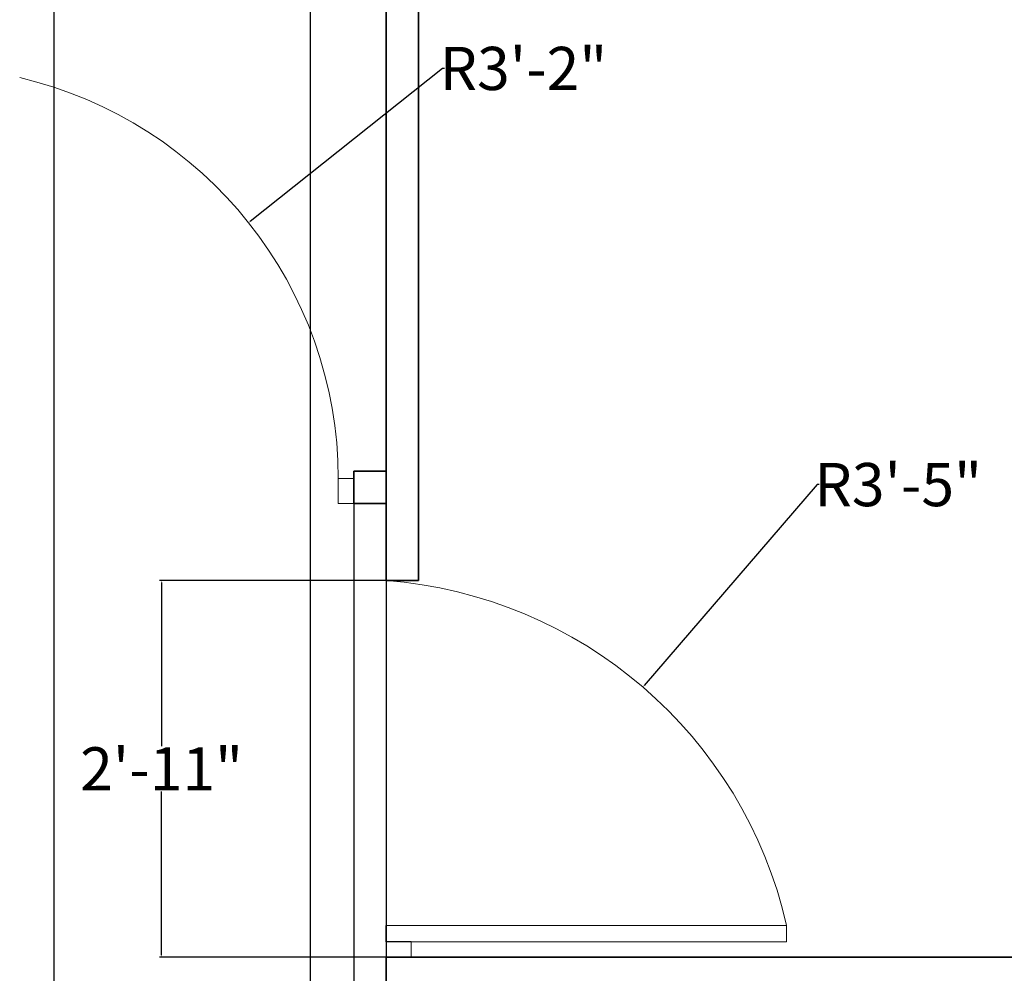
# Model space of a CAD drawing. Units: inches. Extents: x 311 to 754, y 60 to 497.
# Tile 9 of 11: x 530 to 621, y 296 to 384. Entities that reach past the tile are written whole.
import ezdxf

# ---------------------------------------------------------------- set-up
doc = ezdxf.new("R2010")
doc.units = ezdxf.units.IN
doc.header["$MEASUREMENT"] = 0
for name, color, linetype, lineweight in [('A-ANNO-DIMS', 2, 'Continuous', 18), ('A-WALL', 7, 'Continuous', 35), ('beds', 70, 'Continuous', 13), ('doors', 210, 'Continuous', 18)]:
    doc.layers.add(name, color=color, linetype=linetype, lineweight=lineweight)
doc.styles.get("Standard").update_dxf_attribs({"font": 'arial.ttf'})
doc.dimstyles.get("Standard").update_dxf_attribs({"dimtxt": 4, "dimasz": 0.18, "dimexe": 0.18, "dimexo": 0.0625, "dimgap": 0.09, "dimtad": 0, "dimtih": 1, "dimtoh": 1, "dimdec": 0, "dimrnd": 6, "dimzin": 0, "dimdsep": 46, "dimlunit": 3, "dimtxsty": 'Standard', "dimcen": 0.09, "dimadec": 0, "dimazin": 0, "dimtfac": 1, "dimtdec": 0, "dimtofl": 0, "dimtmove": 0, "dimatfit": 3, "dimfxl": 1, "dimtolj": 1, "dimtzin": 0, "dimarcsym": 0})

# ---------------------------------------------------------------- blocks, each defined once
blk = doc.blocks.new('A$C57792D97')
for p, q in [((0.6, 2.6235), (0, 2.6235)), ((0, 2.6235), (0, 2.1735)), ((2.1, 2.6235), (0.6, 2.6235)), ((0.6, 2.6235), (0.6, 0.6235)), ((0.6, 0.6235), (0.6, 2.6235)), ((0.6, 2.1735), (0.6, 2.6235)), ((2.1, 0.6235), (2.1, 2.6235)), ((2.7, 2.6235), (2.1, 2.6235)), ((2.1, 2.6235), (2.1, 2.1735)), ((2.7, 2.1735), (2.7, 2.6235)), ((0.6, 2.5735), (0, 2.5735)), ((2.1, 2.5735), (0.6, 2.5735)), ((2.7, 2.5735), (2.1, 2.5735)), ((2.4103, 2.2312), (2.4103, 2.5317)), ((2.2593, 2.3802), (2.5698, 2.3802)), ((1.5491, 2.1955), (1.5516, 2.1955)), ((0, 2.1735), (0.6, 2.1735)), ((2.1, 2.1735), (2.7, 2.1735)), ((0.6, 2.1518), (0.8661, 2.1518)), ((0.6, 1.9518), (1.4767, 1.9518)), ((0.63, 0.6535), (0.63, 1.9518)), ((0.9906, 1.8942), (0.9508, 1.934)), ((1.4149, 1.8942), (1.3751, 1.934)), ((0.9906, 1.8942), (0.9344, 1.8942)), ((0.9906, 1.8942), (0.9508, 1.8544)), ((1.4149, 1.8942), (1.3586, 1.8942)), ((1.4149, 1.8942), (1.3751, 1.8544)), ((2.142, 1.8959), (2.1018, 1.8254)), ((2.1679, 1.8652), (2.1088, 1.8077)), ((2.1584, 1.8544), (2.1201, 1.8188)), ((2.1812, 1.8524), (2.1207, 1.8046)), ((2.1749, 1.8475), (2.1394, 1.7993)), ((2.2173, 1.8274), (2.1931, 1.7688)), ((2.2496, 1.8292), (2.2008, 1.7642)), ((2.1799, 1.8155), (2.1465, 1.7971)), ((2.2066, 1.8191), (2.1664, 1.7827)), ((2.249, 1.8154), (2.1711, 1.7709)), ((2.2713, 1.7954), (2.2055, 1.7458)), ((2.07, 1.7793), (2.07, 0.6535)), ((2.283, 1.7811), (2.2169, 1.7413)), ((2.2607, 1.7859), (2.2181, 1.7554)), ((2.2761, 1.777), (2.2348, 1.7337)), ((2.277, 1.7446), (2.2416, 1.7306)), ((2.304, 1.7449), (2.2596, 1.7138)), ((2.3456, 1.7359), (2.2627, 1.7015)), ((2.3157, 1.7518), (2.2843, 1.6966)), ((2.3479, 1.7495), (2.2914, 1.6911)), ((0.7785, 1.6821), (0.7387, 1.7219)), ((1.2027, 1.6821), (1.163, 1.7219)), ((1.627, 1.6821), (1.5872, 1.7219)), ((2.0513, 1.6821), (2.0115, 1.7219)), ((2.3653, 1.7133), (2.2937, 1.6723)), ((2.3535, 1.7051), (2.3075, 1.6802)), ((0.7785, 1.6821), (0.7222, 1.6821)), ((0.7785, 1.6821), (0.7387, 1.6423)), ((1.2027, 1.6821), (1.1465, 1.6821)), ((1.2027, 1.6821), (1.163, 1.6423)), ((1.627, 1.6821), (1.5708, 1.6821)), ((1.627, 1.6821), (1.5872, 1.6423)), ((2.0513, 1.6821), (1.995, 1.6821)), ((2.0513, 1.6821), (2.0115, 1.6423)), ((2.3751, 1.6976), (2.3045, 1.6664)), ((2.3677, 1.6944), (2.3213, 1.6565)), ((2.3645, 1.6621), (2.3277, 1.6526)), ((2.3913, 1.659), (2.3434, 1.6337)), ((2.4314, 1.6449), (2.3449, 1.6211)), ((2.4038, 1.6644), (2.3657, 1.6136)), ((2.4355, 1.6581), (2.372, 1.6073)), ((2.4482, 1.62), (2.372, 1.5882)), ((2.4354, 1.6134), (2.3867, 1.5944)), ((2.2754, 1.598), (2.2534, 1.5939)), ((2.2736, 1.5771), (2.2535, 1.594)), ((2.2736, 1.5771), (2.2754, 1.598)), ((2.4559, 1.6032), (2.382, 1.581)), ((2.4482, 1.6009), (2.3974, 1.5692)), ((2.3123, 1.541), (2.2911, 1.5481)), ((2.3006, 1.5236), (2.2912, 1.5481)), ((2.441, 1.5693), (2.4032, 1.5645)), ((2.4672, 1.5629), (2.4164, 1.5438)), ((2.4802, 1.5667), (2.4361, 1.5211)), ((2.5109, 1.5564), (2.4416, 1.514)), ((2.3006, 1.5236), (2.3123, 1.541)), ((2.5052, 1.5438), (2.4164, 1.5311)), ((2.5187, 1.517), (2.4392, 1.4951)), ((0.9906, 1.47), (0.9508, 1.5097)), ((1.4149, 1.47), (1.3751, 1.5097)), ((1.8391, 1.47), (1.7994, 1.5097)), ((2.5243, 1.4994), (2.4482, 1.4867)), ((2.5052, 1.5121), (2.4545, 1.4994)), ((2.5163, 1.4981), (2.462, 1.473)), ((0.9906, 1.47), (0.9344, 1.47)), ((0.9906, 1.47), (0.9508, 1.4302)), ((1.4149, 1.47), (1.3586, 1.47)), ((1.4149, 1.47), (1.3751, 1.4302)), ((1.8391, 1.47), (1.7829, 1.47)), ((1.8391, 1.47), (1.7994, 1.4302)), ((2.5052, 1.4677), (2.4672, 1.4677)), ((2.5304, 1.458), (2.4777, 1.4454)), ((2.5438, 1.4601), (2.4943, 1.4204)), ((2.5658, 1.4343), (2.4761, 1.4328)), ((2.573, 1.4461), (2.4989, 1.4127)), ((2.5758, 1.406), (2.4942, 1.3942)), ((2.5618, 1.4028), (2.5099, 1.3966)), ((2.5791, 1.3878), (2.502, 1.3848)), ((2.571, 1.3876), (2.514, 1.3695)), ((2.1596, 1.3147), (2.1502, 1.3392)), ((2.1714, 1.3321), (2.1502, 1.3392)), ((2.2534, 1.3469), (2.2315, 1.3429)), ((2.2516, 1.326), (2.2315, 1.3429)), ((2.2516, 1.326), (2.2535, 1.347)), ((2.5562, 1.3587), (2.5185, 1.3635)), ((2.58, 1.346), (2.5261, 1.3402)), ((2.5936, 1.3464), (2.5395, 1.3132)), ((2.1596, 1.3147), (2.1714, 1.3321)), ((2.3632, 1.3229), (2.33, 1.319)), ((2.3584, 1.2918), (2.33, 1.319)), ((2.3584, 1.2918), (2.3632, 1.3229)), ((2.6121, 1.3181), (2.523, 1.3279)), ((2.6207, 1.3289), (2.5431, 1.305)), ((0.7785, 1.2578), (0.7387, 1.2976)), ((1.2027, 1.2578), (1.163, 1.2976)), ((1.627, 1.2578), (1.5872, 1.2976)), ((2.0513, 1.2578), (2.0115, 1.2976)), ((2.6185, 1.2888), (2.5361, 1.2873)), ((2.6195, 1.2703), (2.5426, 1.277)), ((2.6042, 1.2873), (2.5519, 1.2877)), ((0.7785, 1.2578), (0.7222, 1.2578)), ((0.7785, 1.2578), (0.7387, 1.218)), ((1.2027, 1.2578), (1.1465, 1.2578)), ((1.2027, 1.2578), (1.163, 1.218)), ((1.627, 1.2578), (1.5708, 1.2578)), ((1.627, 1.2578), (1.5872, 1.218)), ((2.0513, 1.2578), (1.995, 1.2578)), ((2.0513, 1.2578), (2.0115, 1.218)), ((2.4134, 1.2295), (2.404, 1.254)), ((2.4252, 1.2469), (2.404, 1.254)), ((2.4134, 1.2295), (2.4252, 1.2469)), ((2.6115, 1.2711), (2.5526, 1.2603)), ((2.5932, 1.2443), (2.5563, 1.2538)), ((2.6435, 1.197), (2.5563, 1.2178)), ((2.6152, 1.2287), (2.561, 1.2296)), ((2.6287, 1.2274), (2.5709, 1.2013)), ((2.6534, 1.2066), (2.5734, 1.1926)), ((2.6462, 1.1671), (2.5642, 1.176)), ((2.6449, 1.1486), (2.5694, 1.1649)), ((2.6319, 1.1675), (2.58, 1.1743)), ((2.4947, 1.1445), (2.4728, 1.1404)), ((2.4929, 1.1236), (2.4728, 1.1404)), ((2.4929, 1.1236), (2.4948, 1.1445)), ((2.637, 1.1504), (2.5773, 1.147)), ((2.6155, 1.1261), (2.5801, 1.1402)), ((2.2315, 1.0959), (2.2095, 1.0919)), ((2.2297, 1.075), (2.2315, 1.0959)), ((2.6595, 1.0729), (2.5756, 1.1045)), ((2.6353, 1.1079), (2.5817, 1.1156)), ((2.6486, 1.1049), (2.588, 1.0862)), ((0.9906, 1.0457), (0.9508, 1.0855)), ((1.4149, 1.0457), (1.3751, 1.0855)), ((1.8391, 1.0457), (1.7994, 1.0855)), ((2.2297, 1.075), (2.2096, 1.0919)), ((2.6584, 1.0429), (2.5782, 1.062)), ((2.6705, 1.0812), (2.5894, 1.0774)), ((0.9906, 1.0457), (0.9344, 1.0457)), ((0.9906, 1.0457), (0.9508, 1.0059)), ((1.4149, 1.0457), (1.3586, 1.0457)), ((1.4149, 1.0457), (1.3751, 1.0059)), ((1.8391, 1.0457), (1.7829, 1.0457)), ((1.8391, 1.0457), (1.7994, 1.0059)), ((2.2725, 1.0206), (2.2631, 1.0451)), ((2.2842, 1.038), (2.2631, 1.0451)), ((2.2725, 1.0206), (2.2843, 1.038)), ((2.6548, 1.0248), (2.582, 1.0503)), ((2.6472, 1.0275), (2.5875, 1.0316)), ((2.6442, 1.045), (2.5937, 1.0584)), ((2.6228, 1.0061), (2.5895, 1.0244)), ((2.6598, 0.9477), (2.5805, 0.9897)), ((2.6402, 0.9855), (2.588, 0.9999)), ((2.653, 0.9809), (2.5905, 0.97)), ((2.3053, 0.9493), (2.272, 0.9455)), ((2.3005, 0.9182), (2.2721, 0.9455)), ((2.3005, 0.9182), (2.3053, 0.9494)), ((2.5263, 0.9355), (2.5169, 0.96)), ((2.538, 0.9528), (2.5169, 0.9599)), ((2.5263, 0.9355), (2.5381, 0.9529)), ((2.655, 0.9181), (2.5778, 0.9471)), ((2.6718, 0.9546), (2.5908, 0.961)), ((2.6412, 0.9221), (2.5927, 0.9416)), ((2.6491, 0.9006), (2.5801, 0.9351)), ((2.6419, 0.9043), (2.5832, 0.9159)), ((2.4728, 0.8934), (2.4508, 0.8894)), ((2.471, 0.8725), (2.4509, 0.8894)), ((2.471, 0.8725), (2.4728, 0.8934)), ((2.6297, 0.8635), (2.5797, 0.8843)), ((2.6151, 0.8861), (2.5843, 0.9085)), ((0.7785, 0.8336), (0.7387, 0.8733)), ((1.2027, 0.8336), (1.163, 0.8733)), ((1.627, 0.8336), (1.5872, 0.8733)), ((2.0513, 0.8336), (2.0115, 0.8733)), ((2.6444, 0.8236), (2.571, 0.8751)), ((2.6418, 0.8573), (2.5785, 0.8543)), ((0.7785, 0.8336), (0.7222, 0.8336)), ((0.7785, 0.8336), (0.7387, 0.7938)), ((1.2027, 0.8336), (1.1465, 0.8336)), ((1.2027, 0.8336), (1.163, 0.7938)), ((1.627, 0.8336), (1.5708, 0.8336)), ((1.627, 0.8336), (1.5872, 0.7938)), ((2.0513, 0.8336), (1.995, 0.8336)), ((2.0513, 0.8336), (2.0115, 0.7938)), ((2.1316, 0.8117), (2.1222, 0.8362)), ((2.1433, 0.8291), (2.1222, 0.8362)), ((2.1316, 0.8117), (2.1434, 0.8291)), ((2.2095, 0.8449), (2.1876, 0.8408)), ((2.2077, 0.824), (2.1876, 0.8408)), ((2.2077, 0.824), (2.2095, 0.8449)), ((2.6359, 0.7948), (2.5629, 0.8332)), ((2.6279, 0.7781), (2.5637, 0.821)), ((2.6227, 0.8004), (2.577, 0.8259)), ((2.6572, 0.8289), (2.5776, 0.8454)), ((1.9462, 0.7963), (1.9243, 0.7923)), ((2.6212, 0.7827), (2.5644, 0.8015)), ((2.5923, 0.768), (2.5646, 0.7941)), ((2.6136, 0.7023), (2.5472, 0.7626)), ((2.604, 0.7437), (2.557, 0.7707)), ((1.683, 0.7477), (1.661, 0.7437)), ((2.3854, 0.7265), (2.376, 0.751)), ((2.3971, 0.7439), (2.376, 0.751)), ((2.3854, 0.7265), (2.3972, 0.7439)), ((2.6269, 0.706), (2.5501, 0.7323)), ((2.6153, 0.7361), (2.552, 0.7411)), ((1.4197, 0.6992), (1.3978, 0.6951)), ((2.5915, 0.6593), (2.5332, 0.7099)), ((2.6016, 0.6748), (2.534, 0.7221)), ((2.5892, 0.6821), (2.547, 0.7131)), ((2.5549, 0.6537), (2.5307, 0.6831)), ((2.5855, 0.6646), (2.5315, 0.6905)), ((0.9906, 0.6214), (0.9508, 0.6612)), ((1.1564, 0.6506), (1.1345, 0.6466)), ((1.4149, 0.6214), (1.3751, 0.6612)), ((1.8391, 0.6214), (1.7994, 0.6612)), ((2.4508, 0.6424), (2.4289, 0.6383)), ((2.449, 0.6215), (2.4289, 0.6384)), ((2.449, 0.6215), (2.4508, 0.6424)), ((2.5678, 0.5858), (2.5095, 0.654)), ((2.5635, 0.6282), (2.5203, 0.6608)), ((0.9906, 0.6214), (0.9344, 0.6214)), ((0.9906, 0.6214), (0.9727, 0.6035)), ((1.4149, 0.6214), (1.3586, 0.6214)), ((1.4149, 0.6214), (1.397, 0.6035)), ((1.8391, 0.6214), (1.7829, 0.6214)), ((1.8391, 0.6214), (1.8212, 0.6035)), ((2.5524, 0.5601), (2.4913, 0.6155)), ((2.5815, 0.5878), (2.5085, 0.6236)), ((2.5737, 0.6192), (2.5116, 0.632)), ((2.02, 0.6035), (0.6716, 0.6035)), ((0.8932, 0.6021), (0.8712, 0.598)), ((2.1875, 0.5938), (2.1656, 0.5898)), ((2.1857, 0.5729), (2.1656, 0.5898)), ((2.1857, 0.5729), (2.1876, 0.5938)), ((2.5035, 0.545), (2.4831, 0.5772)), ((2.5352, 0.552), (2.4849, 0.5844)), ((2.5405, 0.546), (2.489, 0.6034)), ((2.541, 0.5688), (2.5031, 0.6049)), ((0.6417, 0.5735), (2.05, 0.5735)), ((1.3422, 0.5642), (1.3386, 0.5735)), ((1.3422, 0.5642), (1.3485, 0.5735)), ((2.2473, 0.5758), (2.2141, 0.5719)), ((2.2425, 0.5447), (2.2141, 0.572)), ((2.2425, 0.5447), (2.2474, 0.5758)), ((2.5078, 0.476), (2.4585, 0.551)), ((2.5088, 0.5186), (2.47, 0.5564)), ((0.8062, 0.5164), (0.8823, 0.5291)), ((0.8118, 0.4988), (0.8913, 0.5207)), ((0.8142, 0.5177), (0.8685, 0.5428)), ((0.8253, 0.5037), (0.876, 0.5164)), ((1.8485, 0.5294), (1.8152, 0.5255)), ((1.8437, 0.4983), (1.8153, 0.5256)), ((1.8437, 0.4983), (1.8485, 0.5294)), ((1.9243, 0.5453), (1.9023, 0.5412)), ((1.9225, 0.5244), (1.9024, 0.5412)), ((1.9225, 0.5244), (1.9243, 0.5453)), ((2.2445, 0.5176), (2.2351, 0.5421)), ((2.2445, 0.5176), (2.2562, 0.535)), ((2.5216, 0.4763), (2.4537, 0.5209)), ((2.5178, 0.5084), (2.4578, 0.5289)), ((0.8196, 0.4594), (0.8889, 0.5018)), ((0.8503, 0.4491), (0.8944, 0.4947)), ((1.6077, 0.4964), (1.5865, 0.5035)), ((1.596, 0.479), (1.5866, 0.5035)), ((1.596, 0.479), (1.6077, 0.4964)), ((1.661, 0.4967), (1.6391, 0.4927)), ((1.6592, 0.4758), (1.6391, 0.4927)), ((1.6592, 0.4758), (1.661, 0.4967)), ((2.4757, 0.4399), (2.4318, 0.5034)), ((2.4893, 0.4525), (2.4356, 0.515)), ((2.4791, 0.4625), (2.446, 0.503)), ((0.8253, 0.472), (0.9141, 0.4847)), ((0.8633, 0.4529), (0.9141, 0.472)), ((0.9592, 0.4578), (0.938, 0.4649)), ((0.9403, 0.459), (0.9381, 0.4649)), ((0.9508, 0.4454), (0.9592, 0.4578)), ((1.4496, 0.483), (1.4163, 0.4791)), ((1.4448, 0.4519), (1.4164, 0.4792)), ((1.4448, 0.4519), (1.4496, 0.483)), ((2.4345, 0.3746), (2.395, 0.4552)), ((2.4409, 0.4167), (2.4071, 0.4591)), ((2.4389, 0.4436), (2.4227, 0.478)), ((2.4712, 0.4466), (2.4253, 0.485)), ((0.8746, 0.4126), (0.9485, 0.4347)), ((0.8823, 0.4149), (0.9331, 0.4466)), ((0.8823, 0.3958), (0.9585, 0.4275)), ((0.8895, 0.4465), (0.9273, 0.4513)), ((1.0507, 0.4366), (1.0175, 0.4327)), ((1.0459, 0.4055), (1.0175, 0.4328)), ((1.0459, 0.4055), (1.0507, 0.4366)), ((1.3977, 0.4481), (1.3758, 0.4441)), ((1.3959, 0.4272), (1.3758, 0.4441)), ((1.3959, 0.4272), (1.3978, 0.4482)), ((2.4482, 0.3731), (2.3865, 0.4259)), ((2.4485, 0.4055), (2.3915, 0.4334)), ((0.895, 0.3577), (0.9585, 0.4085)), ((0.8951, 0.4024), (0.9438, 0.4214)), ((0.8991, 0.3709), (0.9856, 0.3946)), ((0.9267, 0.3514), (0.9648, 0.4022)), ((1.1345, 0.3996), (1.1125, 0.3955)), ((1.1327, 0.3787), (1.1126, 0.3955)), ((1.1327, 0.3787), (1.1345, 0.3996)), ((1.8615, 0.4113), (1.8403, 0.4184)), ((1.8498, 0.3939), (1.8404, 0.4184)), ((1.8498, 0.3939), (1.8615, 0.4113)), ((2.3981, 0.3428), (2.3625, 0.4113)), ((2.4132, 0.3535), (2.3678, 0.4224)), ((2.4043, 0.3648), (2.3766, 0.4092)), ((0.9392, 0.3568), (0.9872, 0.3821)), ((1.213, 0.3727), (1.1918, 0.3798)), ((1.2013, 0.3553), (1.1919, 0.3798)), ((1.2013, 0.3553), (1.213, 0.3727)), ((2.3491, 0.2832), (2.32, 0.3681)), ((2.3607, 0.3242), (2.3324, 0.3704)), ((2.3621, 0.3511), (2.3503, 0.3873)), ((2.3945, 0.35), (2.3538, 0.3939)), ((0.9555, 0.3182), (1.026, 0.3494)), ((0.9628, 0.3214), (1.0092, 0.3592)), ((0.9652, 0.3025), (1.0368, 0.3435)), ((0.966, 0.3537), (1.0029, 0.3631)), ((0.977, 0.3107), (1.023, 0.3356)), ((2.1656, 0.3428), (2.1436, 0.3387)), ((2.1638, 0.3219), (2.1437, 0.3388)), ((2.1638, 0.3219), (2.1656, 0.3428)), ((2.3253, 0.265), (2.2888, 0.3389)), ((2.3625, 0.28), (2.3078, 0.3401)), ((2.3668, 0.3121), (2.3138, 0.3469)), ((0.9826, 0.2663), (1.0392, 0.3246)), ((0.9849, 0.2799), (1.0678, 0.3143)), ((1.0148, 0.264), (1.0462, 0.3191)), ((2.1153, 0.3261), (2.0941, 0.3332)), ((2.1036, 0.3087), (2.0942, 0.3332)), ((2.1036, 0.3087), (2.1153, 0.3261)), ((2.2743, 0.2689), (2.2671, 0.3063)), ((2.3063, 0.2638), (2.2714, 0.3124)), ((2.309, 0.2562), (2.2823, 0.3286)), ((2.3179, 0.2773), (2.2959, 0.3247)), ((1.0265, 0.2709), (1.0709, 0.302)), ((1.0475, 0.2347), (1.1136, 0.2745)), ((1.0535, 0.2712), (1.0889, 0.2852)), ((1.0544, 0.2388), (1.0957, 0.2821)), ((1.4668, 0.2875), (1.4456, 0.2946)), ((1.4551, 0.2701), (1.4457, 0.2946)), ((1.4551, 0.2701), (1.4668, 0.2875)), ((1.9023, 0.2942), (1.8804, 0.2902)), ((1.9005, 0.2733), (1.8804, 0.2902)), ((1.9005, 0.2733), (1.9023, 0.2942)), ((2.2529, 0.2032), (2.2346, 0.291)), ((2.2695, 0.2424), (2.2473, 0.2918)), ((1.0592, 0.2203), (1.125, 0.27)), ((1.0699, 0.2299), (1.1124, 0.2604)), ((1.0809, 0.1866), (1.1297, 0.2516)), ((1.0815, 0.2004), (1.1594, 0.2449)), ((1.1132, 0.1884), (1.1374, 0.247)), ((1.639, 0.2457), (1.6171, 0.2416)), ((1.6372, 0.2248), (1.6391, 0.2457)), ((2.2097, 0.1814), (2.1923, 0.2566)), ((2.227, 0.1881), (2.2001, 0.2661)), ((2.2212, 0.2012), (2.2053, 0.2511)), ((2.2658, 0.1984), (2.2191, 0.2649)), ((2.2741, 0.2296), (2.2258, 0.2708)), ((1.1239, 0.1967), (1.1641, 0.2331)), ((1.1507, 0.2003), (1.184, 0.2187)), ((1.1556, 0.1683), (1.1911, 0.2165)), ((1.6372, 0.2248), (1.6171, 0.2416)), ((2.1474, 0.1359), (2.1403, 0.2253)), ((2.1688, 0.1727), (2.1529, 0.2245)), ((2.1768, 0.1984), (2.1745, 0.2364)), ((2.208, 0.1893), (2.1795, 0.2419)), ((1.1493, 0.1634), (1.2098, 0.2112)), ((1.1626, 0.1506), (1.2217, 0.2081)), ((1.1721, 0.1614), (1.2104, 0.197)), ((1.1873, 0.1336), (1.259, 0.1875)), ((1.1885, 0.1199), (1.2287, 0.1904)), ((1.2203, 0.1256), (1.237, 0.1868)), ((1.3758, 0.1971), (1.3538, 0.193)), ((1.374, 0.1762), (1.3539, 0.1931)), ((1.374, 0.1762), (1.3758, 0.1971)), ((1.7206, 0.2023), (1.6994, 0.2094)), ((1.7089, 0.1849), (1.6995, 0.2095)), ((1.7089, 0.1849), (1.7206, 0.2024)), ((2.1011, 0.1277), (2.0794, 0.1835)), ((2.1018, 0.1197), (2.0939, 0.1965)), ((2.1198, 0.1242), (2.1029, 0.2049)), ((2.1157, 0.1379), (2.1062, 0.1893)), ((2.1596, 0.1295), (2.1216, 0.2013)), ((2.1718, 0.1594), (2.129, 0.2063)), ((1.2299, 0.1352), (1.2652, 0.1764)), ((1.2559, 0.1422), (1.2867, 0.1646)), ((1.2592, 0.1054), (1.3133, 0.1604)), ((1.2649, 0.111), (1.2941, 0.1633)), ((1.2741, 0.0944), (1.3255, 0.1588)), ((1.7905, 0.1559), (1.7573, 0.152)), ((1.7857, 0.1248), (1.7573, 0.152)), ((1.7857, 0.1248), (1.7906, 0.1559)), ((2.0054, 0.0742), (1.9988, 0.1564)), ((2.0614, 0.1027), (2.0249, 0.1545)), ((2.0343, 0.0824), (2.0385, 0.172)), ((2.0601, 0.1162), (2.0509, 0.1696)), ((2.0714, 0.1407), (2.0737, 0.1787)), ((1.282, 0.1063), (1.3156, 0.1464)), ((1.3007, 0.0806), (1.3651, 0.1431)), ((1.3035, 0.0671), (1.3346, 0.1421)), ((1.3344, 0.0768), (1.3433, 0.1396)), ((1.3427, 0.0876), (1.3725, 0.1328)), ((1.3677, 0.0977), (1.3954, 0.1238)), ((1.3755, 0.0616), (1.4223, 0.1229)), ((1.3804, 0.0679), (1.4028, 0.1234)), ((1.3916, 0.0525), (1.4346, 0.1229)), ((1.9154, 0.0434), (1.9307, 0.1318)), ((1.9452, 0.0737), (1.9428, 0.1279)), ((1.9595, 0.0966), (1.9666, 0.134)), ((1.9873, 0.08), (1.9728, 0.1381)), ((1.9871, 0.072), (1.9889, 0.1491)), ((2.0031, 0.0883), (2.0001, 0.1405)), ((2.0456, 0.0745), (2.0169, 0.1505)), ((1.3981, 0.0653), (1.4264, 0.1093)), ((1.4198, 0.0422), (1.4758, 0.1123)), ((1.4243, 0.0292), (1.4458, 0.1075)), ((1.4537, 0.0427), (1.4546, 0.1061)), ((1.4606, 0.0544), (1.4845, 0.103)), ((1.4841, 0.0676), (1.5083, 0.0969)), ((1.4964, 0.0327), (1.5351, 0.0995)), ((1.5005, 0.0397), (1.5158, 0.0975)), ((1.5135, 0.0258), (1.5473, 0.101)), ((1.5428, 0.0191), (1.5896, 0.0956)), ((1.6378, 0.0145), (1.6619, 0.0934)), ((1.6677, 0.0115), (1.7045, 0.0933)), ((1.7442, 0.0214), (1.7651, 0.0956)), ((1.7625, 0.0189), (1.7765, 0.1002)), ((1.7925, 0.0197), (1.8188, 0.1054)), ((1.8238, 0.0326), (1.8014, 0.0919)), ((1.8259, 0.046), (1.8303, 0.1)), ((1.8429, 0.0669), (1.8547, 0.1031)), ((1.8685, 0.047), (1.8614, 0.1064)), ((1.8672, 0.039), (1.8787, 0.1154)), ((1.8852, 0.0532), (1.8888, 0.1054)), ((1.8857, 0.0389), (1.8894, 0.1213)), ((1.9256, 0.0342), (1.9067, 0.1132)), ((1.9448, 0.0601), (1.9151, 0.1162)), ((1.5183, 0.0393), (1.5409, 0.0865)), ((1.5489, 0.0067), (1.5603, 0.0871)), ((1.5763, 0.0238), (1.5693, 0.0868)), ((1.5817, 0.0362), (1.5994, 0.0875)), ((1.6034, 0.0523), (1.6237, 0.0845)), ((1.6199, 0.0192), (1.65, 0.0903)), ((1.6232, 0.0266), (1.631, 0.086)), ((1.6409, 0.0285), (1.6573, 0.0782)), ((1.6753, 0), (1.6766, 0.0812)), ((1.7004, 0.0204), (1.6855, 0.0821)), ((1.7041, 0.0334), (1.7152, 0.0865)), ((1.7236, 0.0521), (1.7398, 0.0865)), ((1.7465, 0.0291), (1.7469, 0.0889)), ((1.7638, 0.0332), (1.7739, 0.0845)), ((1.8015, 0.0092), (1.7926, 0.09))]:
    blk.add_line(p, q)
at = {"linetype": 'ByBlock'}
for p, q in [((0.3217, 2.5511), (0.3189, 2.5483)), ((0.5475, 2.5511), (0.3217, 2.5511)), ((0.5475, 2.5511), (0.5503, 2.5483)), ((0.3189, 2.5483), (0.3189, 2.3511)), ((0.3375, 2.5469), (0.3303, 2.5397)), ((0.3303, 2.5397), (0.3303, 2.3683)), ((0.3346, 2.5426), (0.3332, 2.5369)), ((0.3332, 2.5369), (0.3332, 2.4983)), ((0.3332, 2.5369), (0.346, 2.524)), ((0.3403, 2.5454), (0.3346, 2.5426)), ((0.3803, 2.5469), (0.3375, 2.5469)), ((0.3746, 2.5454), (0.3403, 2.5454)), ((0.3475, 2.5269), (0.3403, 2.5454)), ((0.346, 2.524), (0.3475, 2.5269)), ((0.346, 2.4597), (0.346, 2.524)), ((0.3475, 2.5269), (0.3675, 2.5269)), ((0.3675, 2.5269), (0.3746, 2.5454)), ((0.3689, 2.524), (0.3675, 2.5269)), ((0.3818, 2.5369), (0.3689, 2.524)), ((0.3689, 2.4597), (0.3689, 2.524)), ((0.3746, 2.5454), (0.3803, 2.5426)), ((0.386, 2.5397), (0.3803, 2.5469)), ((0.3803, 2.5426), (0.3818, 2.5369)), ((0.3818, 2.5369), (0.3818, 2.4983)), ((0.386, 2.3668), (0.386, 2.5397)), ((0.3989, 2.4597), (0.3989, 2.5354)), ((0.3989, 2.5354), (0.5418, 2.5354)), ((0.5418, 2.5354), (0.5418, 2.4597)), ((0.5503, 2.5483), (0.5503, 2.3511)), ((0.3332, 2.4983), (0.336, 2.4911)), ((0.336, 2.4911), (0.3403, 2.484)), ((0.3789, 2.4911), (0.3746, 2.484)), ((0.3818, 2.4983), (0.3789, 2.4911)), ((0.3403, 2.484), (0.3417, 2.474)), ((0.3417, 2.474), (0.3417, 2.4597)), ((0.3417, 2.4326), (0.3417, 2.4597)), ((0.346, 2.4597), (0.346, 2.3826)), ((0.3689, 2.4597), (0.3689, 2.3826)), ((0.3746, 2.484), (0.3732, 2.474)), ((0.3732, 2.474), (0.3732, 2.4597)), ((0.3732, 2.4326), (0.3732, 2.4597)), ((0.5418, 2.4597), (0.3989, 2.4597)), ((0.3403, 2.4226), (0.3417, 2.4326)), ((0.3746, 2.4226), (0.3732, 2.4326)), ((0.3989, 2.4426), (0.3989, 2.4568)), ((0.3989, 2.4568), (0.5361, 2.4568)), ((0.5361, 2.4426), (0.3989, 2.4426)), ((0.4675, 2.4568), (0.4675, 2.4426)), ((0.4789, 2.4568), (0.4789, 2.4426)), ((0.4903, 2.4568), (0.4903, 2.4426)), ((0.5018, 2.4568), (0.5018, 2.4426)), ((0.5132, 2.4568), (0.5132, 2.4426)), ((0.5246, 2.4568), (0.5246, 2.4426)), ((0.5361, 2.4568), (0.5361, 2.4426)), ((0.3332, 2.4083), (0.336, 2.4154)), ((0.3332, 2.3697), (0.3332, 2.4083)), ((0.336, 2.4154), (0.3403, 2.4226)), ((0.3789, 2.4154), (0.3746, 2.4226)), ((0.3818, 2.4083), (0.3789, 2.4154)), ((0.3818, 2.3697), (0.3818, 2.4083)), ((0.3989, 2.4197), (0.3989, 2.4111)), ((0.4103, 2.4197), (0.3989, 2.4197)), ((0.3989, 2.4111), (0.4103, 2.4111)), ((0.3989, 2.404), (0.3989, 2.3954)), ((0.4103, 2.404), (0.3989, 2.404)), ((0.4103, 2.4111), (0.4103, 2.4197)), ((0.4103, 2.3954), (0.4103, 2.404)), ((0.4275, 2.4197), (0.416, 2.4197)), ((0.416, 2.4197), (0.416, 2.4111)), ((0.416, 2.4111), (0.4275, 2.4111)), ((0.416, 2.404), (0.416, 2.3954)), ((0.4275, 2.404), (0.416, 2.404)), ((0.4275, 2.4111), (0.4275, 2.4197)), ((0.4275, 2.3954), (0.4275, 2.404)), ((0.4332, 2.4197), (0.4332, 2.4111)), ((0.4446, 2.4197), (0.4332, 2.4197)), ((0.4332, 2.4111), (0.4446, 2.4111)), ((0.4332, 2.404), (0.4332, 2.3954)), ((0.4446, 2.404), (0.4332, 2.404)), ((0.4446, 2.4111), (0.4446, 2.4197)), ((0.4446, 2.3954), (0.4446, 2.404)), ((0.4575, 2.4011), (0.4575, 2.4268)), ((0.4575, 2.4268), (0.5418, 2.4268)), ((0.5418, 2.4011), (0.4575, 2.4011)), ((0.4718, 2.424), (0.4761, 2.424)), ((0.4718, 2.4197), (0.4718, 2.424)), ((0.4761, 2.4197), (0.4718, 2.4197)), ((0.4718, 2.4083), (0.4761, 2.4083)), ((0.4718, 2.404), (0.4718, 2.4083)), ((0.4761, 2.404), (0.4718, 2.404)), ((0.4761, 2.424), (0.4761, 2.4197)), ((0.4761, 2.4083), (0.4761, 2.404)), ((0.4975, 2.424), (0.5018, 2.424)), ((0.4975, 2.4197), (0.4975, 2.424)), ((0.5018, 2.4197), (0.4975, 2.4197)), ((0.4975, 2.4083), (0.5018, 2.4083)), ((0.4975, 2.404), (0.4975, 2.4083)), ((0.5018, 2.404), (0.4975, 2.404)), ((0.5018, 2.424), (0.5018, 2.4197)), ((0.5018, 2.4083), (0.5018, 2.404)), ((0.5232, 2.4197), (0.5232, 2.424)), ((0.5232, 2.424), (0.5275, 2.424)), ((0.5275, 2.4197), (0.5232, 2.4197)), ((0.5232, 2.4083), (0.5275, 2.4083)), ((0.5232, 2.404), (0.5232, 2.4083)), ((0.5275, 2.404), (0.5232, 2.404)), ((0.5275, 2.424), (0.5275, 2.4197)), ((0.5275, 2.4083), (0.5275, 2.404)), ((0.5418, 2.4268), (0.5418, 2.4011)), ((0.2955, 2.3663), (0.298, 2.3689)), ((0.298, 2.3689), (0.3033, 2.3669)), ((0.3033, 2.3669), (0.3063, 2.3696)), ((0.3063, 2.3696), (0.3103, 2.3737)), ((0.3126, 2.3694), (0.3068, 2.3648)), ((0.3103, 2.3737), (0.3189, 2.3768)), ((0.3189, 2.3711), (0.3126, 2.3694)), ((0.3303, 2.3683), (0.3375, 2.3597)), ((0.3332, 2.3697), (0.346, 2.3826)), ((0.3346, 2.364), (0.3332, 2.3697)), ((0.3475, 2.3797), (0.3403, 2.3611)), ((0.346, 2.3826), (0.3475, 2.3797)), ((0.3475, 2.3797), (0.3675, 2.3797)), ((0.3689, 2.3826), (0.3675, 2.3797)), ((0.3675, 2.3797), (0.3746, 2.3611)), ((0.3818, 2.3697), (0.3689, 2.3826)), ((0.3789, 2.3597), (0.386, 2.3668)), ((0.3803, 2.364), (0.3818, 2.3697)), ((0.3989, 2.3954), (0.4103, 2.3954)), ((0.4103, 2.3883), (0.3989, 2.3883)), ((0.3989, 2.3883), (0.3989, 2.3797)), ((0.3989, 2.3797), (0.4103, 2.3797)), ((0.4103, 2.3711), (0.3989, 2.3711)), ((0.3989, 2.3711), (0.3989, 2.3626)), ((0.4103, 2.3797), (0.4103, 2.3883)), ((0.4103, 2.3626), (0.4103, 2.3711)), ((0.416, 2.3954), (0.4275, 2.3954)), ((0.4275, 2.3868), (0.416, 2.3868)), ((0.416, 2.3868), (0.416, 2.3783)), ((0.416, 2.3783), (0.4275, 2.3783)), ((0.416, 2.3711), (0.416, 2.3626)), ((0.4275, 2.3711), (0.416, 2.3711)), ((0.4275, 2.3783), (0.4275, 2.3868)), ((0.4275, 2.3626), (0.4275, 2.3711)), ((0.4332, 2.3954), (0.4446, 2.3954)), ((0.4446, 2.3868), (0.4332, 2.3868)), ((0.4332, 2.3868), (0.4332, 2.3783)), ((0.4332, 2.3783), (0.4446, 2.3783)), ((0.4332, 2.3711), (0.4332, 2.3626)), ((0.4446, 2.3711), (0.4332, 2.3711)), ((0.4446, 2.3783), (0.4446, 2.3868)), ((0.4446, 2.3626), (0.4446, 2.3711)), ((0.4661, 2.394), (0.4803, 2.394)), ((0.4661, 2.3883), (0.4661, 2.394)), ((0.4803, 2.3883), (0.4661, 2.3883)), ((0.4661, 2.3726), (0.4661, 2.364)), ((0.4803, 2.3726), (0.4661, 2.3726)), ((0.4803, 2.394), (0.4803, 2.3883)), ((0.4803, 2.364), (0.4803, 2.3726)), ((0.4861, 2.3883), (0.4861, 2.394)), ((0.4861, 2.394), (0.5003, 2.394)), ((0.5003, 2.3883), (0.4861, 2.3883)), ((0.5003, 2.3726), (0.4861, 2.3726)), ((0.4861, 2.3726), (0.4861, 2.364)), ((0.5003, 2.394), (0.5003, 2.3883)), ((0.5003, 2.364), (0.5003, 2.3726)), ((0.5061, 2.3883), (0.5061, 2.394)), ((0.5061, 2.394), (0.5203, 2.394)), ((0.5203, 2.3883), (0.5061, 2.3883)), ((0.5203, 2.3726), (0.5061, 2.3726)), ((0.5061, 2.3726), (0.5061, 2.364)), ((0.5203, 2.394), (0.5203, 2.3883)), ((0.5203, 2.364), (0.5203, 2.3726)), ((0.5261, 2.3883), (0.5261, 2.394)), ((0.5261, 2.394), (0.5403, 2.394)), ((0.5403, 2.3883), (0.5261, 2.3883)), ((0.5403, 2.3726), (0.5261, 2.3726)), ((0.5261, 2.3726), (0.5261, 2.364)), ((0.5403, 2.394), (0.5403, 2.3883)), ((0.5403, 2.364), (0.5403, 2.3726)), ((0.2683, 2.3394), (0.2738, 2.3452)), ((0.2706, 2.3331), (0.2683, 2.3394)), ((0.2738, 2.3452), (0.2804, 2.3412)), ((0.2937, 2.3497), (0.2748, 2.3336)), ((0.2789, 2.3502), (0.2854, 2.3565)), ((0.2804, 2.3412), (0.2789, 2.3502)), ((0.2854, 2.3565), (0.2932, 2.3525)), ((0.2902, 2.3608), (0.294, 2.3648)), ((0.2932, 2.3525), (0.2902, 2.3608)), ((0.3053, 2.3601), (0.2937, 2.3497)), ((0.294, 2.3648), (0.2975, 2.3621)), ((0.2975, 2.3621), (0.2955, 2.3663)), ((0.3053, 2.3628), (0.3023, 2.3631)), ((0.3023, 2.3631), (0.3053, 2.3601)), ((0.3068, 2.3648), (0.3053, 2.3628)), ((0.3189, 2.3511), (0.3217, 2.3483)), ((0.3217, 2.3483), (0.3525, 2.3483)), ((0.3403, 2.3611), (0.3346, 2.364)), ((0.3375, 2.3597), (0.3542, 2.3597)), ((0.3543, 2.3611), (0.3403, 2.3611)), ((0.3483, 2.3311), (0.3518, 2.3447)), ((0.3518, 2.3447), (0.3538, 2.354)), ((0.3552, 2.3386), (0.3518, 2.325)), ((0.3538, 2.354), (0.3546, 2.3654)), ((0.3546, 2.3654), (0.3589, 2.3654)), ((0.3587, 2.3531), (0.3552, 2.3386)), ((0.3575, 2.3483), (0.5475, 2.3483)), ((0.3589, 2.3654), (0.3587, 2.3531)), ((0.3746, 2.3611), (0.3588, 2.3611)), ((0.3588, 2.3597), (0.3789, 2.3597)), ((0.3746, 2.3611), (0.3803, 2.364)), ((0.3989, 2.3626), (0.4103, 2.3626)), ((0.416, 2.3626), (0.4275, 2.3626)), ((0.4332, 2.3626), (0.4446, 2.3626)), ((0.4661, 2.364), (0.4803, 2.364)), ((0.4861, 2.364), (0.5003, 2.364)), ((0.5061, 2.364), (0.5203, 2.364)), ((0.5261, 2.364), (0.5403, 2.364)), ((0.5503, 2.3511), (0.5475, 2.3483)), ((0.2532, 2.3027), (0.2546, 2.31)), ((0.2546, 2.31), (0.2624, 2.31)), ((0.2563, 2.3158), (0.2584, 2.3224)), ((0.2624, 2.31), (0.2563, 2.3158)), ((0.2584, 2.3224), (0.2676, 2.3221)), ((0.2592, 2.3253), (0.2618, 2.334)), ((0.2676, 2.3221), (0.2592, 2.3253)), ((0.2618, 2.334), (0.2705, 2.3331)), ((0.2746, 2.3331), (0.265, 2.3059)), ((0.265, 2.3059), (0.2691, 2.2842)), ((0.3422, 2.288), (0.3437, 2.3062)), ((0.3425, 2.3129), (0.3477, 2.3166)), ((0.3437, 2.3062), (0.3425, 2.3129)), ((0.3474, 2.3242), (0.3483, 2.3311)), ((0.3477, 2.3166), (0.3474, 2.3242)), ((0.352, 2.3175), (0.3512, 2.3158)), ((0.3512, 2.3158), (0.3544, 2.3126)), ((0.3518, 2.325), (0.352, 2.3175)), ((0.3544, 2.3126), (0.3549, 2.3056)), ((0.2621, 2.3001), (0.2532, 2.3027)), ((0.2546, 2.2958), (0.2621, 2.3001)), ((0.2558, 2.29), (0.2546, 2.2958)), ((0.2647, 2.2903), (0.2558, 2.29)), ((0.2578, 2.2825), (0.2647, 2.2903)), ((0.2601, 2.2767), (0.2578, 2.2825)), ((0.2685, 2.2793), (0.2601, 2.2767)), ((0.2644, 2.2715), (0.2685, 2.2793)), ((0.2691, 2.2842), (0.2818, 2.2718)), ((0.3312, 2.2741), (0.3422, 2.288)), ((0.3492, 2.2776), (0.3405, 2.2793)), ((0.3405, 2.2793), (0.3445, 2.2712)), ((0.3541, 2.2915), (0.3448, 2.2906)), ((0.3448, 2.2906), (0.3529, 2.2842)), ((0.3549, 2.3056), (0.3466, 2.3042)), ((0.3466, 2.3042), (0.3546, 2.2993)), ((0.3529, 2.2842), (0.3492, 2.2776)), ((0.3546, 2.2993), (0.3541, 2.2915)), ((0.2682, 2.268), (0.2644, 2.2715)), ((0.2763, 2.2715), (0.2682, 2.268)), ((0.2728, 2.2637), (0.2763, 2.2715)), ((0.2774, 2.2596), (0.2728, 2.2637)), ((0.2835, 2.2672), (0.2774, 2.2596)), ((0.2818, 2.2718), (0.2986, 2.2646)), ((0.2827, 2.2585), (0.2835, 2.2672)), ((0.2873, 2.2562), (0.2827, 2.2585)), ((0.2939, 2.262), (0.2873, 2.2562)), ((0.2942, 2.2541), (0.2939, 2.262)), ((0.2997, 2.2527), (0.2942, 2.2541)), ((0.2986, 2.2646), (0.3159, 2.266)), ((0.3029, 2.262), (0.2997, 2.2527)), ((0.3049, 2.2536), (0.3029, 2.262)), ((0.3098, 2.2541), (0.3049, 2.2536)), ((0.3133, 2.262), (0.3098, 2.2541)), ((0.3171, 2.2541), (0.3133, 2.262)), ((0.3159, 2.266), (0.3312, 2.2741)), ((0.3231, 2.2559), (0.3171, 2.2541)), ((0.3292, 2.2596), (0.3223, 2.2654)), ((0.3223, 2.2654), (0.3231, 2.2559)), ((0.3347, 2.2631), (0.3292, 2.2596)), ((0.3402, 2.266), (0.3335, 2.2709)), ((0.3335, 2.2709), (0.3347, 2.2631)), ((0.3445, 2.2712), (0.3402, 2.266))]:
    blk.add_line(p, q, dxfattribs=at)
for centre, radius in [((2.4068, 2.3792), 0.1082), ((2.4128, 2.3792), 0.062)]:
    blk.add_circle(centre, radius)
for centre, radius, start, end in [((0.8117, 1.4495), 1.1155, 75.3755, 98.4519), ((0.7133, 2.123), 0.4349, 62.6153, 98.6623), ((0.9995, 2.5566), 0.3518, 180.6066, 203.849), ((1.5803, 0.4369), 2.1259, 84.0997, 95.547), ((7.229, 2.8402), 5.8612, 182.80995, 184.16642), ((2.0384, 6.4739), 3.9297, 266.5056, 270.1818), ((1.2711, 1.6927), 0.8548, 85.0132, 101.9962), ((0.9942, 1.5092), 1.0245, 76.8495, 84.445), ((-2.6554, 2.4937), 4.0011, 355.9906, 0.7251), ((1.505, 1.754), 0.7941, 71.9705, 99.0452), ((1.6997, 1.5092), 1.0245, 76.8495, 84.445), ((2.5231, 2.3654), 0.505, 159.2551, 197.4606), ((6.5168, 1.1676), 5.2262, 165.6998, 168.4122), ((1.7461, 2.3905), 1.0686, 178.7205, 189.3246), ((2.4516, 2.3905), 1.0686, 178.7205, 189.3246), ((1.0382, 2.187), 0.3479, 146.8128, 174.9884), ((1.3553, 2.3447), 0.1322, 217.4973, 261.5591), ((2.6076, 3.8927), 1.7717, 246.8027, 251.3608), ((0.9964, 4.7934), 2.5939, 263.2521, 270.4789), ((1.5587, 3.1365), 0.9332, 260.0314, 280.1788), ((1.8907, 2.8521), 0.6558, 255.2386, 283.2855), ((1.1218, 3.4256), 1.2305, 265.1643, 280.0187), ((1.0153, 0.392), 1.7661, 72.4208, 94.846), ((0.7898, 0.8867), 1.2674, 53.0057, 86.5496), ((2.0108, 3.233), 1.2462, 248.2311, 274.1028), ((1.991, 2.6169), 0.8413, 238.5747, 277.4412), ((1.6653, 1.0079), 0.9493, 207.2312, 62.7432), ((1.6653, 1.0079), 0.9093, 208.5361, 61.4369), ((0.6787, 0.6517), 0.0487, 177.8916, 261.664), ((2.02, 0.6535), 0.05, 270, 0), ((0.6518, 0.6244), 0.0518, 180.9151, 258.7324), ((2.05, 0.6235), 0.05, 270, 0)]:
    blk.add_arc(centre, radius, start, end)
blk = doc.blocks.new('*D130')
at = {"layer": 'A-ANNO-DIMS', "color": 0, "lineweight": -2, "transparency": 16777216}
for p, q in [((563.742, 332.098), (542.825, 332.098)), ((543.005, 331.918), (543.005, 316.766)), ((543.005, 297.418), (543.005, 312.57)), ((563.742, 297.238), (542.825, 297.238))]:
    blk.add_line(p, q, dxfattribs=at)
at = {"layer": 'A-ANNO-DIMS', "color": 0, "transparency": 16777216}
for points in [[(542.975, 331.918), (543.035, 331.918), (543.005, 332.098)], [(542.975, 297.418), (543.035, 297.418), (543.005, 297.238)]]:
    blk.add_solid(points, dxfattribs=at)
at = {"layer": 'Defpoints', "color": 0, "transparency": 16777216}
for p in [(543.005, 332.098), (563.805, 332.098), (563.805, 297.238)]:
    blk.add_point(p, dxfattribs=at)
at = {"layer": 'A-ANNO-DIMS', "color": 0, "transparency": 16777216, "insert": (543.005, 314.668), "char_height": 4, "attachment_point": 5}
blk.add_mtext('\\A1;2\'-11"', dxfattribs=at)
blk = doc.blocks.new('*D132')
at = {"layer": 'A-ANNO-DIMS', "color": 0, "lineweight": -2, "transparency": 16777216}
for p, q in [((526.906, 339.175), (526.906, 66.258)), ((560.824, 339.175), (560.824, 66.258)), ((527.086, 66.438), (536.871, 66.438)), ((560.644, 66.438), (550.86, 66.438))]:
    blk.add_line(p, q, dxfattribs=at)
at = {"layer": 'A-ANNO-DIMS', "color": 0, "transparency": 16777216}
for points in [[(527.086, 66.468), (527.086, 66.408), (526.906, 66.438)], [(560.644, 66.468), (560.644, 66.408), (560.824, 66.438)]]:
    blk.add_solid(points, dxfattribs=at)
at = {"layer": 'Defpoints', "color": 0, "transparency": 16777216}
for p in [(526.906, 339.238), (560.824, 339.238), (526.906, 66.438)]:
    blk.add_point(p, dxfattribs=at)
at = {"layer": 'A-ANNO-DIMS', "color": 0, "transparency": 16777216, "insert": (543.865, 66.438), "char_height": 4, "attachment_point": 5}
blk.add_mtext('\\A1;2\'-10"', dxfattribs=at)
blk = doc.blocks.new('*D134')
at = {"layer": 'A-ANNO-DIMS', "color": 0, "lineweight": -2, "transparency": 16777216}
for p, q in [((494.805, 342.175), (494.805, 66.258)), ((563.805, 342.175), (563.805, 66.258)), ((494.985, 66.438), (523.898, 66.438)), ((563.625, 66.438), (534.711, 66.438))]:
    blk.add_line(p, q, dxfattribs=at)
at = {"layer": 'A-ANNO-DIMS', "color": 0, "transparency": 16777216}
for points in [[(494.985, 66.468), (494.985, 66.408), (494.805, 66.438)], [(563.625, 66.468), (563.625, 66.408), (563.805, 66.438)]]:
    blk.add_solid(points, dxfattribs=at)
at = {"layer": 'Defpoints', "color": 0, "transparency": 16777216}
for p in [(494.805, 342.238), (563.805, 342.238), (563.805, 66.438)]:
    blk.add_point(p, dxfattribs=at)
at = {"layer": 'A-ANNO-DIMS', "color": 0, "transparency": 16777216, "insert": (529.305, 66.438), "char_height": 4, "attachment_point": 5}
blk.add_mtext('\\A1;5\'-9"', dxfattribs=at)
blk = doc.blocks.new('*D146')
at = {"layer": 'A-ANNO-DIMS', "color": 0, "lineweight": -2, "transparency": 16777216}
for p, q in [((533.038, 385.855), (533.038, 66.258)), ((556.776, 385.855), (556.776, 66.258)), ((533.218, 66.438), (533.474, 66.438)), ((556.596, 66.438), (556.339, 66.438))]:
    blk.add_line(p, q, dxfattribs=at)
at = {"layer": 'A-ANNO-DIMS', "color": 0, "transparency": 16777216}
for points in [[(533.218, 66.468), (533.218, 66.408), (533.038, 66.438)], [(556.596, 66.468), (556.596, 66.408), (556.776, 66.438)]]:
    blk.add_solid(points, dxfattribs=at)
at = {"layer": 'Defpoints', "color": 0, "transparency": 16777216}
for p in [(533.038, 385.917), (556.776, 385.917), (556.776, 66.438)]:
    blk.add_point(p, dxfattribs=at)
at = {"layer": 'A-ANNO-DIMS', "color": 0, "transparency": 16777216, "insert": (544.907, 66.438), "char_height": 4, "attachment_point": 5}
blk.add_mtext('\\A1;1\'-11 1/2"', dxfattribs=at)
blk = doc.blocks.new('*D154')
at = {"layer": 'A-ANNO-DIMS', "color": 0, "lineweight": -2, "transparency": 16777216}
for p, q in [((603.74, 340.986), (587.717, 322.369)), ((603.92, 340.986), (603.74, 340.986)), ((560.61, 290.978), (560.79, 290.978)), ((560.7, 290.888), (560.7, 291.068))]:
    blk.add_line(p, q, dxfattribs=at)
at = {"layer": 'A-ANNO-DIMS', "color": 0, "transparency": 16777216}
blk.add_solid([(587.695, 322.389), (587.74, 322.35), (587.6, 322.233)], dxfattribs=at)
at = {"layer": 'Defpoints', "color": 0, "transparency": 16777216}
for p in [(587.6, 322.233), (560.7, 290.978)]:
    blk.add_point(p, dxfattribs=at)
at = {"layer": 'A-ANNO-DIMS', "color": 0, "transparency": 16777216, "insert": (611.241, 340.986), "char_height": 4, "attachment_point": 5}
blk.add_mtext('\\A1;R3\'-5"', dxfattribs=at)
blk = doc.blocks.new('*D155')
at = {"layer": 'A-ANNO-DIMS', "color": 0, "lineweight": -2, "transparency": 16777216}
for p, q in [((569.026, 379.515), (551.209, 365.347)), ((569.206, 379.515), (569.026, 379.515)), ((521.05, 341.435), (521.23, 341.435)), ((521.14, 341.345), (521.14, 341.525))]:
    blk.add_line(p, q, dxfattribs=at)
at = {"layer": 'A-ANNO-DIMS', "color": 0, "transparency": 16777216}
blk.add_solid([(551.191, 365.37), (551.228, 365.323), (551.069, 365.235)], dxfattribs=at)
at = {"layer": 'Defpoints', "color": 0, "transparency": 16777216}
for p in [(551.069, 365.235), (521.14, 341.435)]:
    blk.add_point(p, dxfattribs=at)
at = {"layer": 'A-ANNO-DIMS', "color": 0, "transparency": 16777216, "insert": (576.526, 379.515), "char_height": 4, "attachment_point": 5}
blk.add_mtext('\\A1;R3\'-2"', dxfattribs=at)

msp = doc.modelspace()

# ---------------------------------------------------------------- linework, layer by layer
at = {"layer": 'A-WALL'}
for p, q in [((563.805, 342.238), (563.805, 438.238)), ((566.805, 332.098), (566.805, 438.238)), ((563.805, 342.238), (560.824, 342.238)), ((560.824, 342.238), (560.824, 339.238)), ((563.805, 342.238), (560.824, 342.238)), ((563.805, 342.238), (563.805, 339.238)), ((563.805, 339.238), (560.824, 339.238)), ((563.805, 332.098), (563.805, 339.238)), ((563.805, 332.098), (566.805, 332.098)), ((713.805, 297.238), (563.805, 297.238)), ((563.805, 231.238), (563.805, 297.238))]:
    msp.add_line(p, q, dxfattribs=at)
at = {"layer": 'doors'}
for points in [[(559.378, 339.238), (560.824, 339.238), (560.824, 341.551), (559.378, 341.551)], [(563.785, 300.173), (563.785, 298.651), (600.899, 298.651), (600.899, 300.173)], [(563.804, 298.684), (563.804, 297.238), (566.117, 297.238), (566.117, 298.684)]]:
    msp.add_lwpolyline(points, close=True, dxfattribs=at)
for centre, radius, start, end in [((521.14, 341.435), 38.238, 0.17407, 76.81095), ((560.7, 290.978), 41.237, 12.88392, 85.68231)]:
    msp.add_arc(centre, radius, start, end, dxfattribs=at)

# ---------------------------------------------------------------- block references
at = {"layer": 'beds', "xscale": 30.06046351726443, "yscale": 30.06046351726443, "zscale": 30.06046351726443}
msp.add_blockref('A$C57792D97', (613.186, 352.32), dxfattribs=at)

# ---------------------------------------------------------------- dimensions: what is measured, and where the dimension line sits
at = {"layer": 'A-ANNO-DIMS'}
for base, p1, p2, picture, middle in [((556.776, 66.438), (533.038, 385.917), (556.776, 385.917), '*D146', (544.907, 66.438)), ((563.805, 66.438), (494.805, 342.238), (563.805, 342.238), '*D134', (529.305, 66.438)), ((526.906, 66.438), (560.824, 339.238), (526.906, 339.238), '*D132', (543.865, 66.438))]:
    dim = msp.add_linear_dim(base=base, p1=p1, p2=p2, dimstyle='Standard', override={"dimdec": 1, "dimlfac": 1, "dimrnd": 0, "dimzin": 1, "dimdsep": 46, "dimlunit": 4, "dimfrac": 2}, dxfattribs=at)
    dim.commit()
    dim.dimension.update_dxf_attribs({"geometry": picture, "text_midpoint": middle})
for center, mpoint, picture, middle in [((521.14, 341.435), (551.069, 365.235), '*D155', (576.526, 379.515)), ((560.7, 290.978), (587.6, 322.233), '*D154', (611.241, 340.986))]:
    dim = msp.add_radius_dim(center=center, mpoint=mpoint, dimstyle='Standard', override={"dimdec": 1, "dimlfac": 1, "dimrnd": 0, "dimzin": 1, "dimdsep": 46, "dimlunit": 4, "dimfrac": 2}, dxfattribs=at)
    dim.commit()
    dim.dimension.update_dxf_attribs({"geometry": picture, "text_midpoint": middle, "dimtype": 164})
dim = msp.add_linear_dim(base=(543.005, 332.098), p1=(563.805, 297.238), p2=(563.805, 332.098), angle=90, dimstyle='Standard', override={"dimdec": 1, "dimlfac": 1, "dimrnd": 0, "dimzin": 1, "dimdsep": 46, "dimlunit": 4, "dimfrac": 2}, dxfattribs=at)
dim.commit()
dim.dimension.update_dxf_attribs({"geometry": '*D130', "text_midpoint": (543.005, 314.668)})

doc.saveas('drawing.dxf')
